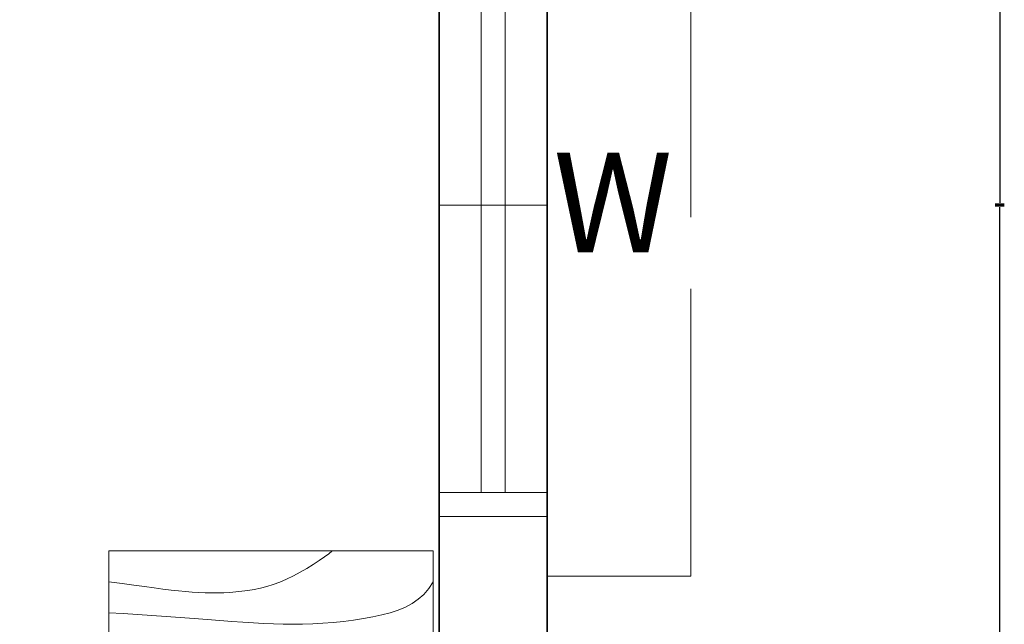
# Model space of a CAD drawing. Units: inches. Extents: x -128 to 854, y -395 to 398.
# Tile 37 of 61: x 270 to 352, y 95 to 145. Entities that reach past the tile are written whole.
import ezdxf

# ---------------------------------------------------------------- set-up
doc = ezdxf.new("R2010")
doc.units = ezdxf.units.IN
doc.header["$MEASUREMENT"] = 0
doc.linetypes.add('ACAD_ISO02W100', pattern=[15, 12, -3])
for name, color, linetype, lineweight in [('A-ANNO-DIMS', 2, 'Continuous', 18), ('A-ANNO-TEXT', 2, 'Continuous', 18), ('A-FURN', 8, 'Continuous', 18), ('A-GLAZ', 220, 'Continuous', 18), ('A-GLAZ-OVHD', 220, 'ACAD_ISO02W100', 13), ('A-WALL', 4, 'Continuous', 35)]:
    doc.layers.add(name, color=color, linetype=linetype, lineweight=lineweight)
doc.styles.get("Standard").update_dxf_attribs({"font": 'arial.ttf'})
doc.dimstyles.get("Standard").update_dxf_attribs({"dimtxt": 0.18, "dimasz": 0.18, "dimexe": 0.18, "dimexo": 0.0625, "dimgap": 0.09, "dimtad": 0, "dimtih": 1, "dimtoh": 1, "dimdec": 1, "dimzin": 0, "dimdsep": 46, "dimlunit": 4, "dimtxsty": 'Standard', "dimcen": 0.09, "dimclrd": 1, "dimclre": 2, "dimclrt": 6, "dimadec": 0, "dimazin": 0, "dimtfac": 1, "dimtdec": 1, "dimtofl": 0, "dimtmove": 0, "dimatfit": 3, "dimfxl": 1, "dimtfill": 2, "dimtfillclr": 3, "dimtolj": 1, "dimtzin": 0, "dimarcsym": 0})

# ---------------------------------------------------------------- blocks, each defined once
blk = doc.blocks.new('Table - Square Woodgrain 42 x 42 in.')
blk.add_line((0, -42), (42, -42))
for points in [[(0, -4), (1.704, -4.2172), (3.2358, -4.4188), (4.615, -4.604), (5.8615, -4.7721), (6.9951, -4.9224), (8.0357, -5.0541), (9.0031, -5.1667), (9.9171, -5.2594), (10.7951, -5.3316), (11.6445, -5.3836), (12.4702, -5.4157), (13.277, -5.4283), (14.0698, -5.4217), (14.8535, -5.3964), (15.6331, -5.3526), (16.4133, -5.2908), (17.1986, -5.2103), (17.9913, -5.1062), (18.793, -4.9727), (19.6056, -4.8038), (20.4307, -4.5937), (21.2701, -4.3365), (22.1256, -4.0262), (22.9989, -3.6571), (23.888, -3.2272), (24.7756, -2.7516), (25.6408, -2.2491), (26.4624, -1.7387), (27.2195, -1.2395), (27.891, -0.7703), (28.456, -0.3501), (28.8934, 0.002)], [(0, -42), (0, 0), (42, 0), (42, -42)], [(0, -8), (1.8203, -8.1001), (3.6741, -8.2149), (5.5411, -8.3408), (7.4011, -8.4741), (9.2339, -8.6112), (11.0193, -8.7484), (12.7371, -8.8821), (14.3671, -9.0086), (15.8954, -9.1246), (17.3337, -9.2278), (18.6997, -9.3159), (20.0116, -9.387), (21.2871, -9.4389), (22.5442, -9.4696), (23.8008, -9.477), (25.0749, -9.459), (26.3791, -9.4137), (27.7049, -9.3403), (29.0383, -9.2382), (30.3655, -9.1068), (31.6728, -8.9455), (32.9461, -8.7535), (34.1717, -8.5304), (35.3358, -8.2756), (36.4268, -7.9863), (37.443, -7.6521), (38.3849, -7.2603), (39.253, -6.7986), (40.048, -6.2542), (40.7705, -5.6147), (41.421, -4.8674), (42, -4)], [(42, -12), (39.1784, -12.8621), (36.4519, -13.5654), (33.8246, -14.1294), (31.3004, -14.5731), (28.8832, -14.9161), (26.577, -15.1775), (24.3858, -15.3768), (22.3136, -15.5332), (20.3622, -15.6632), (18.5254, -15.7718), (16.7947, -15.8612), (15.1618, -15.9338), (13.6183, -15.9916), (12.1558, -16.0369), (10.7659, -16.0718), (9.4403, -16.0987), (8.1703, -16.1191), (6.9461, -16.1325), (5.7577, -16.1377), (4.595, -16.1335), (3.4479, -16.1188), (2.3064, -16.0924), (1.1604, -16.0532), (0, -16)], [(42, -16), (37.6529, -16.7365), (33.8802, -17.329), (30.6179, -17.7961), (27.8015, -18.1561), (25.3668, -18.4275), (23.2497, -18.6288), (21.3859, -18.7785), (19.7111, -18.8949), (18.1693, -18.9939), (16.7375, -19.0795), (15.401, -19.1534), (14.1449, -19.217), (12.9544, -19.2717), (11.8148, -19.3191), (10.7113, -19.3606), (9.6291, -19.3976), (8.5534, -19.4323), (7.47, -19.4689), (6.3643, -19.5122), (5.222, -19.5672), (4.0288, -19.6386), (2.7703, -19.7313), (1.4321, -19.8501), (0, -20)], [(0, -24), (3.9243, -23.6805), (7.4766, -23.4138), (10.6891, -23.1954), (13.5943, -23.0205), (16.2247, -22.8847), (18.6125, -22.7832), (20.7903, -22.7116), (22.7903, -22.6651), (24.6563, -22.642), (26.4764, -22.6507), (28.35, -22.7024), (30.3766, -22.8084), (32.6555, -22.98), (35.2861, -23.2283), (38.3678, -23.5645), (42, -24)], [(42, -32), (37.392, -31.017), (33.4585, -30.2231), (30.1291, -29.5949), (27.3334, -29.109), (25.0009, -28.742), (23.0612, -28.4707), (21.4439, -28.2716), (20.0786, -28.1215), (18.8998, -28.0002), (17.8609, -27.9014), (16.9206, -27.8219), (16.0371, -27.7588), (15.1691, -27.709), (14.2748, -27.6693), (13.3128, -27.6368), (12.2415, -27.6083), (11.0295, -27.5824), (9.6867, -27.5643), (8.233, -27.5608), (6.6884, -27.5787), (5.0728, -27.6248), (3.4062, -27.7058), (1.7086, -27.8286), (0, -28)], [(0, -32), (5.4026, -32.5358), (9.9494, -33.019), (13.7424, -33.4553), (16.8834, -33.8505), (19.4743, -34.2106), (21.6171, -34.5413), (23.4136, -34.8486), (24.9657, -35.1382), (26.3614, -35.4156), (27.6332, -35.6841), (28.7995, -35.9467), (29.8788, -36.2064), (30.8897, -36.4661), (31.8507, -36.7288), (32.7802, -36.9973), (33.6968, -37.2747), (34.6175, -37.5635), (35.5531, -37.8651), (36.5128, -38.1805), (37.506, -38.5108), (38.5421, -38.8568), (39.6302, -39.2197), (40.7797, -39.6004), (42, -40)], [(0, -36), (3.0098, -36.2857), (5.5354, -36.5643), (7.6368, -36.8359), (9.374, -37.1009), (10.807, -37.3597), (11.9957, -37.6126), (13.0002, -37.8599), (13.8804, -38.102), (14.6874, -38.3393), (15.4365, -38.5729), (16.1338, -38.8041), (16.7858, -39.0341), (17.3987, -39.264), (17.9787, -39.4952), (18.5322, -39.7288), (19.0655, -39.9662), (19.5832, -40.2081), (20.0842, -40.4544), (20.5657, -40.7046), (21.0249, -40.9581), (21.459, -41.2144), (21.8653, -41.4731), (22.2409, -41.7335), (22.5831, -41.9951)]]:
    blk.add_lwpolyline(points)
blk = doc.blocks.new('*D55')
at = {"layer": 'A-ANNO-DIMS', "color": 0, "lineweight": -2, "transparency": 16777216}
for p, q in [((304.81, 186.741), (221.092, 186.741)), ((221.272, 181.741), (221.272, 131.873)), ((221.272, 77.741), (221.272, 127.608)), ((304.81, 72.741), (221.092, 72.741))]:
    blk.add_line(p, q, dxfattribs=at)
at = {"layer": 'A-ANNO-DIMS', "color": 0, "transparency": 16777216}
for points in [[(220.439, 181.741), (222.105, 181.741), (221.272, 186.741)], [(220.439, 77.741), (222.105, 77.741), (221.272, 72.741)]]:
    blk.add_solid(points, dxfattribs=at)
at = {"layer": 'Defpoints', "color": 0, "transparency": 16777216}
for p in [(221.272, 186.741), (304.873, 186.741), (304.873, 72.741)]:
    blk.add_point(p, dxfattribs=at)
at = {"layer": 'A-ANNO-DIMS', "color": 0, "transparency": 16777216, "insert": (221.272, 129.741), "char_height": 4, "attachment_point": 5, "bg_fill": 1, "box_fill_scale": 1.25, "bg_fill_color": 3, "bg_fill_transparency": 0}
blk.add_mtext('\\A1;9\'-6"', dxfattribs=at)
blk = doc.blocks.new('WIN-48IN')
for p, q in [((9, 52), (0, 52)), ((9, 50), (0, 50)), ((3.5, 50), (3.5, 2)), ((5.5, 50), (5.5, 2)), ((9, 26), (0, 26)), ((9, 2), (0, 2)), ((9, 0), (0, 0))]:
    blk.add_line(p, q)
blk = doc.blocks.new('SHADE-48IN')
at = {"ltscale": 2}
for p, q in [((12, 62), (0, 62)), ((0, 0), (0, 62)), ((12, 57), (12, 62)), ((12, 5), (12, 0)), ((12, 0), (0, 0))]:
    blk.add_line(p, q, dxfattribs=at)
blk = doc.blocks.new('*D98')
at = {"layer": 'A-ANNO-DIMS', "color": 2, "lineweight": -2, "transparency": 16777216}
for p, q in [((313.935, 348.741), (351.853, 348.741)), ((313.935, -89.259), (351.853, -89.259))]:
    blk.add_line(p, q, dxfattribs=at)
at = {"layer": 'A-ANNO-DIMS', "color": 1, "lineweight": -2, "transparency": 16777216}
for p, q in [((351.673, 348.561), (351.673, 129.923)), ((351.673, -89.079), (351.673, 129.559))]:
    blk.add_line(p, q, dxfattribs=at)
at = {"layer": 'A-ANNO-DIMS', "color": 1, "transparency": 16777216}
for points in [[(351.643, 348.561), (351.703, 348.561), (351.673, 348.741)], [(351.643, -89.079), (351.703, -89.079), (351.673, -89.259)]]:
    blk.add_solid(points, dxfattribs=at)
at = {"layer": 'Defpoints', "color": 0, "transparency": 16777216}
for p in [(313.873, 348.741), (351.673, 348.741), (313.873, -89.259)]:
    blk.add_point(p, dxfattribs=at)
at = {"layer": 'A-ANNO-DIMS', "color": 6, "transparency": 16777216, "insert": (351.673, 129.741), "char_height": 0.18, "attachment_point": 5, "bg_fill": 1, "box_fill_scale": 1.25, "bg_fill_color": 3, "bg_fill_transparency": 0}
blk.add_mtext('\\A1;36\'-6"', dxfattribs=at)

msp = doc.modelspace()

# ---------------------------------------------------------------- linework, layer by layer
at = {"layer": 'A-WALL'}
for p, q in [((313.873, 348.741), (313.873, -89.259)), ((304.873, 186.741), (304.873, 72.741))]:
    msp.add_line(p, q, dxfattribs=at)

# ---------------------------------------------------------------- block references
at = {"layer": 'A-FURN', "xscale": 0.6449685946951323, "yscale": 0.6449685946951323, "zscale": 0.6449685946951323}
msp.add_blockref('Table - Square Woodgrain 42 x 42 in.', (277.284, 100.856), dxfattribs=at)
at = {"layer": 'A-GLAZ', "extrusion": (0, 0, -1), "zscale": -1}
msp.add_blockref('WIN-48IN', (-313.873, 103.741), dxfattribs=at)
at = {"layer": 'A-GLAZ-OVHD', "extrusion": (0, 0, -1), "zscale": -1}
msp.add_blockref('SHADE-48IN', (-325.873, 98.741), dxfattribs=at)

# ---------------------------------------------------------------- texts
at = {"layer": 'A-ANNO-TEXT'}
msp.add_text('W', height=8.314, dxfattribs=at).set_placement((314.396, 125.795))

# ---------------------------------------------------------------- dimensions: what is measured, and where the dimension line sits
at = {"layer": 'A-ANNO-DIMS'}
for base, p1, p2, override, picture, middle in [((351.673, 348.741), (313.873, -89.259), (313.873, 348.741), {"dimdec": 1, "dimlfac": 1, "dimrnd": 0, "dimzin": 1, "dimdsep": 46, "dimlunit": 4, "dimfrac": 2}, '*D98', (351.673, 129.741)), ((221.272, 186.741), (304.873, 72.741), (304.873, 186.741), {"dimtxt": 4, "dimasz": 5, "dimclrd": 0, "dimclre": 0, "dimclrt": 0}, '*D55', (221.272, 129.741))]:
    dim = msp.add_linear_dim(base=base, p1=p1, p2=p2, angle=90, dimstyle='Standard', override=override, dxfattribs=at)
    dim.commit()
    dim.dimension.update_dxf_attribs({"geometry": picture, "text_midpoint": middle})

doc.saveas('drawing.dxf')
